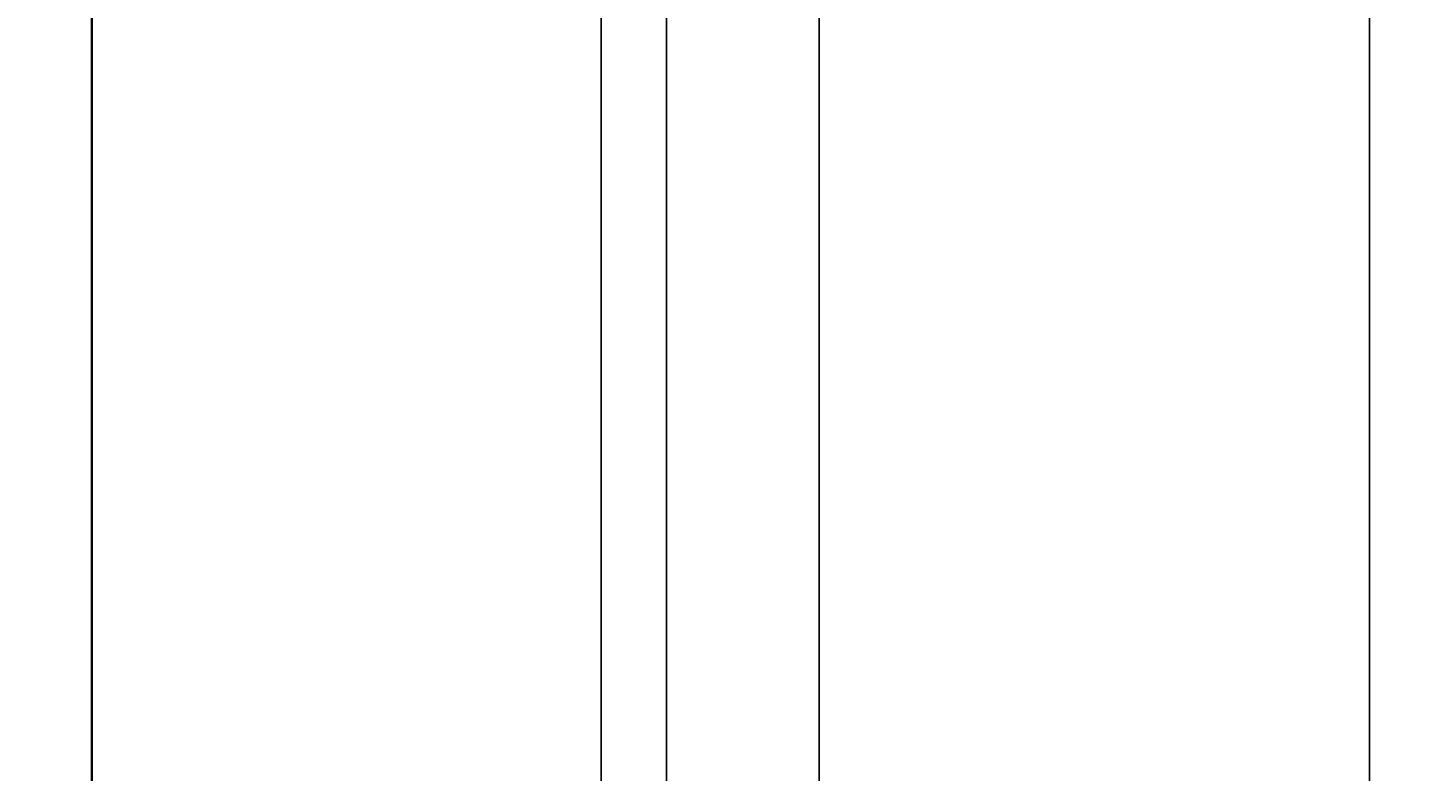
# Model space of a CAD drawing. Units: inches. Extents: x 738 to 1068, y 378 to 757.
# Tile 24 of 41: x 779 to 833, y 549 to 578. Entities that reach past the tile are written whole.
import ezdxf

# ---------------------------------------------------------------- set-up
doc = ezdxf.new("R2010")
doc.units = ezdxf.units.IN
doc.header["$MEASUREMENT"] = 0
doc.layers.add('A-ANNO-DIMS', color=2, linetype='Continuous', lineweight=18)
doc.layers.add('E-POWR-FEED', color=7, linetype='Continuous', lineweight=35)
doc.styles.get("Standard").update_dxf_attribs({"font": 'arial.ttf'})
doc.dimstyles.get("Standard").update_dxf_attribs({"dimtxt": 0.18, "dimasz": 0.18, "dimexe": 0.18, "dimexo": 0.0625, "dimgap": 0.09, "dimtad": 0, "dimtih": 1, "dimtoh": 1, "dimdec": 4, "dimzin": 0, "dimdsep": 46, "dimtxsty": 'Standard', "dimcen": 0.09, "dimadec": 0, "dimazin": 0, "dimtfac": 1, "dimtdec": 4, "dimtofl": 0, "dimtmove": 0, "dimatfit": 3, "dimfxl": 1, "dimtolj": 1, "dimtzin": 0, "dimarcsym": 0})

# ---------------------------------------------------------------- blocks, each defined once
blk = doc.blocks.new('*D22')
at = {"layer": 'A-ANNO-DIMS', "color": 0, "lineweight": -2, "transparency": 16777216}
for p, q in [((781.422, 593.08), (738.194, 593.08)), ((738.374, 592.9), (738.374, 562.422)), ((738.374, 531.581), (738.374, 562.058)), ((781.427, 531.401), (738.194, 531.401))]:
    blk.add_line(p, q, dxfattribs=at)
at = {"layer": 'A-ANNO-DIMS', "color": 0, "transparency": 16777216}
for points in [[(738.344, 592.9), (738.404, 592.9), (738.374, 593.08)], [(738.344, 531.581), (738.404, 531.581), (738.374, 531.401)]]:
    blk.add_solid(points, dxfattribs=at)
at = {"layer": 'Defpoints', "color": 0, "transparency": 16777216}
for p in [(738.374, 593.08), (781.485, 593.08), (781.49, 531.401)]:
    blk.add_point(p, dxfattribs=at)
at = {"layer": 'A-ANNO-DIMS', "color": 0, "transparency": 16777216, "insert": (738.374, 562.24), "char_height": 0.18, "attachment_point": 5}
blk.add_mtext('\\A1;61.68', dxfattribs=at)
blk = doc.blocks.new('*D25')
at = {"layer": 'A-ANNO-DIMS', "color": 0, "lineweight": -2, "transparency": 16777216}
for p, q in [((781.49, 646.923), (781.49, 378.239)), ((803.522, 646.923), (803.522, 378.239)), ((781.67, 378.419), (792.111, 378.419)), ((803.342, 378.419), (792.901, 378.419))]:
    blk.add_line(p, q, dxfattribs=at)
at = {"layer": 'A-ANNO-DIMS', "color": 0, "transparency": 16777216}
for points in [[(781.67, 378.449), (781.67, 378.389), (781.49, 378.419)], [(803.342, 378.449), (803.342, 378.389), (803.522, 378.419)]]:
    blk.add_solid(points, dxfattribs=at)
at = {"layer": 'Defpoints', "color": 0, "transparency": 16777216}
for p in [(781.49, 646.985), (803.522, 646.985), (803.522, 378.419)]:
    blk.add_point(p, dxfattribs=at)
at = {"layer": 'A-ANNO-DIMS', "color": 0, "transparency": 16777216, "insert": (792.506, 378.419), "char_height": 0.18, "attachment_point": 5}
blk.add_mtext('\\A1;22.03', dxfattribs=at)
blk = doc.blocks.new('*D31')
at = {"layer": 'A-ANNO-DIMS', "color": 0, "lineweight": -2, "transparency": 16777216}
for p, q in [((781.49, 531.463), (781.49, 756.505)), ((801.022, 531.463), (801.022, 756.505)), ((781.67, 756.325), (790.802, 756.325)), ((800.842, 756.325), (791.71, 756.325))]:
    blk.add_line(p, q, dxfattribs=at)
at = {"layer": 'A-ANNO-DIMS', "color": 0, "transparency": 16777216}
for points in [[(781.67, 756.355), (781.67, 756.295), (781.49, 756.325)], [(800.842, 756.355), (800.842, 756.295), (801.022, 756.325)]]:
    blk.add_solid(points, dxfattribs=at)
at = {"layer": 'Defpoints', "color": 0, "transparency": 16777216}
for p in [(801.022, 756.325), (781.49, 531.401), (801.022, 531.401)]:
    blk.add_point(p, dxfattribs=at)
at = {"layer": 'A-ANNO-DIMS', "color": 0, "transparency": 16777216, "insert": (791.256, 756.325), "char_height": 0.18, "attachment_point": 5}
blk.add_mtext('\\A1;19.532', dxfattribs=at)
blk = doc.blocks.new('*D32')
at = {"layer": 'A-ANNO-DIMS', "color": 0, "lineweight": -2, "transparency": 16777216}
for p, q in [((809.38, 461.454), (809.38, 756.505)), ((836.232, 461.277), (836.232, 756.505)), ((809.56, 756.325), (822.41, 756.325)), ((836.052, 756.325), (823.202, 756.325))]:
    blk.add_line(p, q, dxfattribs=at)
at = {"layer": 'A-ANNO-DIMS', "color": 0, "transparency": 16777216}
for points in [[(809.56, 756.355), (809.56, 756.295), (809.38, 756.325)], [(836.052, 756.355), (836.052, 756.295), (836.232, 756.325)]]:
    blk.add_solid(points, dxfattribs=at)
at = {"layer": 'Defpoints', "color": 0, "transparency": 16777216}
for p in [(836.232, 756.325), (809.38, 461.392), (836.232, 461.214)]:
    blk.add_point(p, dxfattribs=at)
at = {"layer": 'A-ANNO-DIMS', "color": 0, "transparency": 16777216, "insert": (822.806, 756.325), "char_height": 0.18, "attachment_point": 5}
blk.add_mtext('\\A1;26.85', dxfattribs=at)
blk = doc.blocks.new('*D34')
at = {"layer": 'A-ANNO-DIMS', "color": 0, "lineweight": -2, "transparency": 16777216}
for p, q in [((781.49, 686.266), (781.49, 378.239)), ((830.489, 686.266), (830.489, 378.239)), ((781.67, 378.419), (805.767, 378.419)), ((830.309, 378.419), (806.212, 378.419))]:
    blk.add_line(p, q, dxfattribs=at)
at = {"layer": 'A-ANNO-DIMS', "color": 0, "transparency": 16777216}
for points in [[(781.67, 378.449), (781.67, 378.389), (781.49, 378.419)], [(830.309, 378.449), (830.309, 378.389), (830.489, 378.419)]]:
    blk.add_solid(points, dxfattribs=at)
at = {"layer": 'Defpoints', "color": 0, "transparency": 16777216}
for p in [(781.49, 686.329), (830.489, 686.329), (830.489, 378.419)]:
    blk.add_point(p, dxfattribs=at)
at = {"layer": 'A-ANNO-DIMS', "color": 0, "transparency": 16777216, "insert": (805.99, 378.419), "char_height": 0.18, "attachment_point": 5}
blk.add_mtext('\\A1;49', dxfattribs=at)
blk = doc.blocks.new('*D38')
at = {"layer": 'A-ANNO-DIMS', "color": 0, "lineweight": -2, "transparency": 16777216}
for p, q in [((781.485, 593.017), (781.485, 378.239)), ((887.04, 593.067), (887.04, 378.239)), ((781.665, 378.419), (833.807, 378.419)), ((886.86, 378.419), (834.718, 378.419))]:
    blk.add_line(p, q, dxfattribs=at)
at = {"layer": 'A-ANNO-DIMS', "color": 0, "transparency": 16777216}
for points in [[(781.665, 378.449), (781.665, 378.389), (781.485, 378.419)], [(886.86, 378.449), (886.86, 378.389), (887.04, 378.419)]]:
    blk.add_solid(points, dxfattribs=at)
at = {"layer": 'Defpoints', "color": 0, "transparency": 16777216}
for p in [(781.485, 593.08), (887.04, 593.13), (887.04, 378.419)]:
    blk.add_point(p, dxfattribs=at)
at = {"layer": 'A-ANNO-DIMS', "color": 0, "transparency": 16777216, "insert": (834.263, 378.419), "char_height": 0.18, "attachment_point": 5}
blk.add_mtext('\\A1;105.56', dxfattribs=at)

msp = doc.modelspace()

# ---------------------------------------------------------------- linework, layer by layer
at = {"layer": 'E-POWR-FEED'}
msp.add_line((781.4897, 686.329), (781.4897, 437.7164), dxfattribs=at)

# ---------------------------------------------------------------- dimensions: what is measured, and where the dimension line sits
at = {"layer": 'A-ANNO-DIMS'}
for base, p1, p2, override, picture, middle in [((801.0218, 756.3251), (781.4897, 531.4009), (801.0218, 531.4009), {"dimdec": 3, "dimlfac": 1, "dimrnd": 0, "dimzin": 0, "dimdsep": 46, "dimlunit": 2}, '*D31', (791.2557, 756.3251)), ((836.2324, 756.3251), (809.3803, 461.3919), (836.2324, 461.214), {"dimdec": 2, "dimlfac": 1, "dimrnd": 0, "dimzin": 0, "dimdsep": 46, "dimlunit": 2}, '*D32', (822.8064, 756.3251)), ((830.4893, 378.4191), (781.4897, 686.329), (830.4893, 686.329), {"dimdec": 0, "dimlfac": 1, "dimrnd": 0, "dimzin": 0, "dimdsep": 46, "dimlunit": 2}, '*D34', (805.9895, 378.4191)), ((803.5218, 378.4191), (781.4897, 646.9853), (803.5218, 646.9853), {"dimdec": 2, "dimlfac": 1, "dimrnd": 0, "dimzin": 0, "dimdsep": 46, "dimlunit": 2}, '*D25', (792.5057, 378.4191)), ((887.0404, 378.4191), (781.4846, 593.0796), (887.0404, 593.1296), {"dimdec": 2, "dimlfac": 1, "dimrnd": 0, "dimzin": 0, "dimdsep": 46, "dimlunit": 2}, '*D38', (834.2625, 378.4191))]:
    dim = msp.add_linear_dim(base=base, p1=p1, p2=p2, dimstyle='Standard', override=override, dxfattribs=at)
    dim.commit()
    dim.dimension.update_dxf_attribs({"geometry": picture, "text_midpoint": middle})
dim = msp.add_linear_dim(base=(738.3736, 593.0796), p1=(781.4897, 531.4009), p2=(781.4846, 593.0796), angle=90, dimstyle='Standard', override={"dimdec": 2, "dimlfac": 1, "dimrnd": 0, "dimzin": 0, "dimdsep": 46, "dimlunit": 2}, dxfattribs=at)
dim.commit()
dim.dimension.update_dxf_attribs({"geometry": '*D22', "text_midpoint": (738.3736, 562.2403)})

doc.saveas('drawing.dxf')
